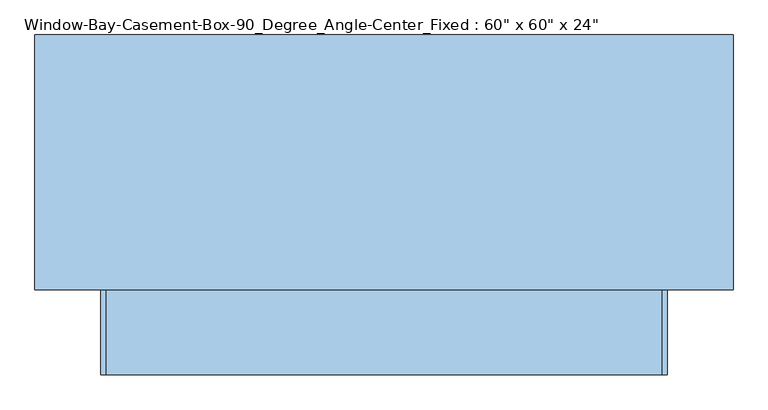
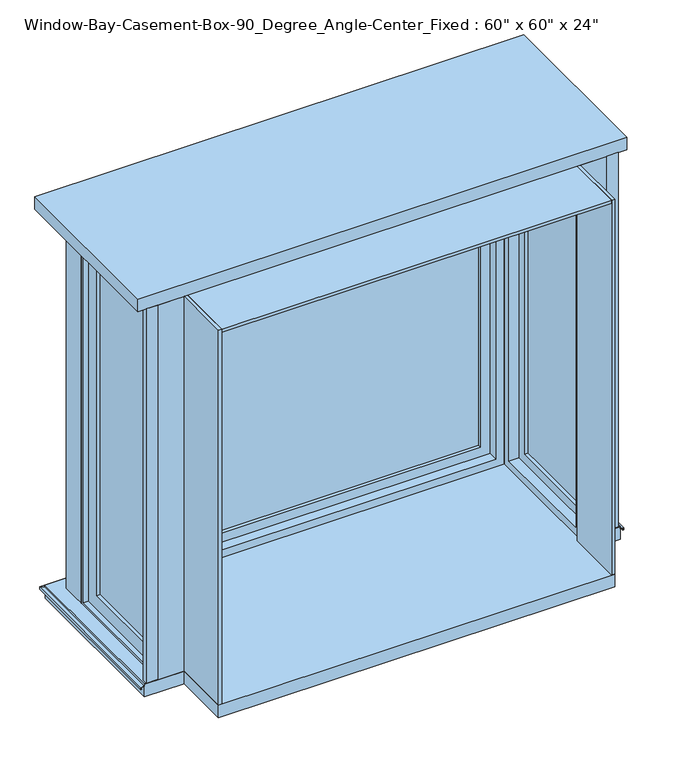
"""IFC4 building model written with IfcOpenShell, lengths in millimetres: window geometry."""

from ifc_helpers import new_model, si_unit, frame, origin, place, context, project, spatial, polyline, outline, extrude, faceted_brep, source, transform, mapped, element, save


def window_dda79932(model_context):
    return source(origin(), model_context, "Body", "SolidModel", [
        extrude(outline(polyline([(-863.6, 114.3), (-908.05, 114.3), (-908.05, 133.35), (-863.6, 133.35), (-863.6, 114.3)])), frame((0.0, 0.0, 663.1486341), z_axis=(0.0, 0.0, 1.0), x_axis=(1.0, 0.0, 0.0)), (0.0, 0.0, 1.0), 1521.2513659),
        extrude(outline(polyline([(908.05, 114.3), (863.6, 114.3), (863.6, 133.35), (908.05, 133.35), (908.05, 114.3)])), frame((0.0, 0.0, 663.1486341), z_axis=(0.0, 0.0, 1.0), x_axis=(1.0, 0.0, 0.0)), (0.0, 0.0, 1.0), 1521.2513659),
        faceted_brep([(-914.4, 114.3, 653.0697935), (-914.4, 114.3, 660.4), (-863.6, 114.3, 660.4), (-863.6, 114.3, 663.1486341), (-915.797, 114.3, 663.1486341), (-915.797, 114.3, 654.4483503), (-928.497, 114.3, 652.2089977), (-928.497, 114.3, 643.2668038), (-924.5346, 114.3, 643.2668038), (-924.5346, 114.3, 644.7270038), (-926.8968, 114.3, 644.7270038), (-926.8968, 114.3, 650.8662705), (914.4, 114.3, 653.0697935), (926.8968, 114.3, 650.8662705), (926.8968, 114.3, 644.7270038), (924.5346, 114.3, 644.7270038), (924.5346, 114.3, 643.2668038), (928.497, 114.3, 643.2668038), (928.497, 114.3, 652.2089977), (915.797, 114.3, 654.4483503), (915.797, 114.3, 663.1486341), (863.6, 114.3, 663.1486341), (863.6, 114.3, 660.4), (914.4, 114.3, 660.4), (-914.4, 774.7, 653.0697935), (-914.4, 774.7, 660.4), (914.4, 774.7, 660.4), (863.6, 723.9, 660.4), (-863.6, 723.9, 660.4), (-863.6, 723.9, 663.1486341), (863.6, 723.9, 663.1486341), (915.797, 776.097, 663.1486341), (-915.797, 776.097, 663.1486341), (-915.797, 776.097, 654.4483503), (-928.497, 788.797, 652.2089977), (-928.497, 788.797, 643.2668038), (928.497, 788.797, 643.2668038), (924.5346, 784.8346, 643.2668038), (-924.5346, 784.8346, 643.2668038), (-924.5346, 784.8346, 644.7270038), (924.5346, 784.8346, 644.7270038), (926.8968, 787.1968, 644.7270038), (-926.8968, 787.1968, 644.7270038), (-926.8968, 787.1968, 650.8662705), (914.4, 774.7, 653.0697935), (915.797, 776.097, 654.4483503), (928.497, 788.797, 652.2089977), (926.8968, 787.1968, 650.8662705)], [[[0, 1, 2, 3, 4, 5, 6, 7, 8, 9, 10, 11]], [[12, 13, 14, 15, 16, 17, 18, 19, 20, 21, 22, 23]], [[1, 0, 24, 25]], [[2, 1, 25, 26, 23, 22, 27, 28]], [[3, 2, 28, 29]], [[4, 3, 29, 30, 21, 20, 31, 32]], [[5, 4, 32, 33]], [[6, 5, 33, 34]], [[7, 6, 34, 35]], [[8, 7, 35, 36, 17, 16, 37, 38]], [[9, 8, 38, 39]], [[10, 9, 39, 40, 15, 14, 41, 42]], [[11, 10, 42, 43]], [[0, 11, 43, 24]], [[25, 24, 44, 26]], [[29, 28, 27, 30]], [[33, 32, 31, 45]], [[34, 33, 45, 46]], [[35, 34, 46, 36]], [[39, 38, 37, 40]], [[43, 42, 41, 47]], [[24, 43, 47, 44]], [[26, 44, 12, 23]], [[30, 27, 22, 21]], [[45, 31, 20, 19]], [[46, 45, 19, 18]], [[36, 46, 18, 17]], [[40, 37, 16, 15]], [[47, 41, 14, 13]], [[44, 47, 13, 12]]]),
        extrude(outline(polyline([(914.4, 774.7), (914.4, 114.3), (762.0, 114.3), (762.0, -114.3), (-762.0, -114.3), (-762.0, 114.3), (-914.4, 114.3), (-914.4, 774.7), (914.4, 774.7)])), frame((0.0, 0.0, 609.6), z_axis=(0.0, 0.0, 1.0), x_axis=(1.0, 0.0, 0.0)), (0.0, 0.0, 1.0), 50.8),
        extrude(outline(polyline([(939.8, 800.1), (939.8, 114.3), (-939.8, 114.3), (-939.8, 800.1), (939.8, 800.1)])), frame((0.0, 0.0, 2184.4), z_axis=(0.0, 0.0, 1.0), x_axis=(1.0, 0.0, 0.0)), (0.0, 0.0, 1.0), 50.8),
        extrude(outline(polyline([(-762.0, 723.9), (-762.0, 622.3), (-863.6, 622.3), (-863.6, 723.9), (-762.0, 723.9)])), frame((0.0, 0.0, 660.4), z_axis=(0.0, 0.0, 1.0), x_axis=(1.0, 0.0, 0.0)), (0.0, 0.0, 1.0), 1524.0),
        extrude(outline(polyline([(863.6, 723.9), (863.6, 622.3), (762.0, 622.3), (762.0, 723.9), (863.6, 723.9)])), frame((0.0, 0.0, 660.4), z_axis=(0.0, 0.0, 1.0), x_axis=(1.0, 0.0, 0.0)), (0.0, 0.0, 1.0), 1524.0),
        faceted_brep([(749.3, 660.4, 673.1), (749.3, 723.9, 673.1), (-749.3, 723.9, 673.1), (-749.3, 660.4, 673.1), (730.25, 622.3, 692.15), (730.25, 660.4, 692.15), (-730.25, 660.4, 692.15), (-730.25, 622.3, 692.15), (762.0, 723.9, 660.4), (762.0, 622.3, 660.4), (-762.0, 622.3, 660.4), (-762.0, 723.9, 660.4), (-749.3, 723.9, 2171.7), (-749.3, 660.4, 2171.7), (-730.25, 660.4, 2152.65), (-730.25, 622.3, 2152.65), (-762.0, 622.3, 2184.4), (-762.0, 723.9, 2184.4), (749.3, 723.9, 2171.7), (749.3, 660.4, 2171.7), (730.25, 660.4, 2152.65), (730.25, 622.3, 2152.65), (762.0, 622.3, 2184.4), (762.0, 723.9, 2184.4)], [[[0, 1, 2, 3]], [[4, 5, 6, 7]], [[8, 9, 10, 11]], [[3, 2, 12, 13]], [[7, 6, 14, 15]], [[11, 10, 16, 17]], [[13, 12, 18, 19]], [[15, 14, 20, 21]], [[17, 16, 22, 23]], [[11, 17, 23, 8], [1, 18, 12, 2]], [[19, 18, 1, 0]], [[3, 13, 19, 0], [5, 20, 14, 6]], [[21, 20, 5, 4]], [[9, 22, 16, 10], [7, 15, 21, 4]], [[23, 22, 9, 8]]]),
        extrude(outline(polyline([(2171.7, -749.3), (673.1, -749.3), (673.1, 749.3), (2171.7, 749.3), (2171.7, -749.3)]), holes=[polyline([(2114.55, 692.15), (730.25, 692.15), (730.25, -692.15), (2114.55, -692.15), (2114.55, 692.15)])]), frame((0.0, 660.4, 0.0), z_axis=(0.0, 1.0, 0.0), x_axis=(0.0, 0.0, 1.0)), (0.0, 0.0, 1.0), 44.45),
        faceted_brep([(-762.0, 146.05, 2152.65), (-800.1, 146.05, 2152.65), (-800.1, 590.55, 2152.65), (-762.0, 590.55, 2152.65), (-863.6, 114.3, 2184.4), (-762.0, 114.3, 2184.4), (-762.0, 622.3, 2184.4), (-863.6, 622.3, 2184.4), (-800.1, 127.0, 2171.7), (-863.6, 127.0, 2171.7), (-863.6, 609.6, 2171.7), (-800.1, 609.6, 2171.7), (-800.1, 590.55, 692.15), (-762.0, 590.55, 692.15), (-762.0, 622.3, 660.4), (-863.6, 622.3, 660.4), (-863.6, 609.6, 673.1), (-800.1, 609.6, 673.1), (-800.1, 146.05, 692.15), (-762.0, 146.05, 692.15), (-762.0, 114.3, 660.4), (-863.6, 114.3, 660.4), (-863.6, 127.0, 673.1), (-800.1, 127.0, 673.1)], [[[0, 1, 2, 3]], [[4, 5, 6, 7]], [[8, 9, 10, 11]], [[3, 2, 12, 13]], [[7, 6, 14, 15]], [[11, 10, 16, 17]], [[13, 12, 18, 19]], [[15, 14, 20, 21]], [[17, 16, 22, 23]], [[11, 17, 23, 8], [1, 18, 12, 2]], [[19, 18, 1, 0]], [[5, 20, 14, 6], [3, 13, 19, 0]], [[21, 20, 5, 4]], [[7, 15, 21, 4], [9, 22, 16, 10]], [[23, 22, 9, 8]]]),
        extrude(outline(polyline([(609.6, 2171.7), (609.6, 673.1), (127.0, 673.1), (127.0, 2171.7), (609.6, 2171.7)]), holes=[polyline([(184.15, 2114.55), (184.15, 730.25), (552.45, 730.25), (552.45, 2114.55), (184.15, 2114.55)])]), frame((-844.55, 0.0, 0.0), z_axis=(1.0, 0.0, 0.0), x_axis=(0.0, 1.0, 0.0)), (0.0, 0.0, 1.0), 44.45),
        faceted_brep([(800.1, 146.05, 2152.65), (762.0, 146.05, 2152.65), (762.0, 590.55, 2152.65), (800.1, 590.55, 2152.65), (863.6, 127.0, 2171.7), (800.1, 127.0, 2171.7), (800.1, 609.6, 2171.7), (863.6, 609.6, 2171.7), (762.0, 114.3, 2184.4), (863.6, 114.3, 2184.4), (863.6, 622.3, 2184.4), (762.0, 622.3, 2184.4), (762.0, 590.55, 692.15), (800.1, 590.55, 692.15), (800.1, 609.6, 673.1), (863.6, 609.6, 673.1), (863.6, 622.3, 660.4), (762.0, 622.3, 660.4), (762.0, 146.05, 692.15), (800.1, 146.05, 692.15), (800.1, 127.0, 673.1), (863.6, 127.0, 673.1), (863.6, 114.3, 660.4), (762.0, 114.3, 660.4)], [[[0, 1, 2, 3]], [[4, 5, 6, 7]], [[8, 9, 10, 11]], [[3, 2, 12, 13]], [[7, 6, 14, 15]], [[11, 10, 16, 17]], [[13, 12, 18, 19]], [[15, 14, 20, 21]], [[17, 16, 22, 23]], [[11, 17, 23, 8], [1, 18, 12, 2]], [[19, 18, 1, 0]], [[5, 20, 14, 6], [3, 13, 19, 0]], [[21, 20, 5, 4]], [[9, 22, 16, 10], [7, 15, 21, 4]], [[23, 22, 9, 8]]]),
        extrude(outline(polyline([(609.6, 2171.7), (609.6, 673.1), (127.0, 673.1), (127.0, 2171.7), (609.6, 2171.7)]), holes=[polyline([(184.15, 2114.55), (184.15, 730.25), (552.45, 730.25), (552.45, 2114.55), (184.15, 2114.55)])]), frame((800.1, 0.0, 0.0), z_axis=(1.0, 0.0, 0.0), x_axis=(0.0, 1.0, 0.0)), (0.0, 0.0, 1.0), 44.45),
        extrude(outline(polyline([(692.15, 692.15), (692.15, 685.8), (-692.15, 685.8), (-692.15, 692.15), (692.15, 692.15)])), frame((0.0, 0.0, 730.25), z_axis=(0.0, 0.0, 1.0), x_axis=(1.0, 0.0, 0.0)), (0.0, 0.0, 1.0), 1384.3),
        extrude(outline(polyline([(692.15, 679.45), (692.15, 673.1), (-692.15, 673.1), (-692.15, 679.45), (692.15, 679.45)])), frame((0.0, 0.0, 730.25), z_axis=(0.0, 0.0, 1.0), x_axis=(1.0, 0.0, 0.0)), (0.0, 0.0, 1.0), 1384.3),
        extrude(outline(polyline([(-825.5, 552.45), (-825.5, 184.15), (-831.85, 184.15), (-831.85, 552.45), (-825.5, 552.45)])), frame((0.0, 0.0, 730.25), z_axis=(0.0, 0.0, 1.0), x_axis=(1.0, 0.0, 0.0)), (0.0, 0.0, 1.0), 1384.3),
        extrude(outline(polyline([(-812.8, 552.45), (-812.8, 184.15), (-819.15, 184.15), (-819.15, 552.45), (-812.8, 552.45)])), frame((0.0, 0.0, 730.25), z_axis=(0.0, 0.0, 1.0), x_axis=(1.0, 0.0, 0.0)), (0.0, 0.0, 1.0), 1384.3),
        extrude(outline(polyline([(831.85, 552.45), (831.85, 184.15), (825.5, 184.15), (825.5, 552.45), (831.85, 552.45)])), frame((0.0, 0.0, 730.25), z_axis=(0.0, 0.0, 1.0), x_axis=(1.0, 0.0, 0.0)), (0.0, 0.0, 1.0), 1384.3),
        extrude(outline(polyline([(819.15, 552.45), (819.15, 184.15), (812.8, 184.15), (812.8, 552.45), (819.15, 552.45)])), frame((0.0, 0.0, 730.25), z_axis=(0.0, 0.0, 1.0), x_axis=(1.0, 0.0, 0.0)), (0.0, 0.0, 1.0), 1384.3),
        faceted_brep([(863.6, 127.0, 2171.7), (800.1, 127.0, 2171.7), (800.1, 609.6, 2171.7), (863.6, 609.6, 2171.7), (762.0, 114.3, 2184.4), (863.6, 114.3, 2184.4), (863.6, 622.3, 2184.4), (762.0, 622.3, 2184.4), (800.1, 146.05, 2152.65), (762.0, 146.05, 2152.65), (762.0, 590.55, 2152.65), (800.1, 590.55, 2152.65), (800.1, 609.6, 673.1), (863.6, 609.6, 673.1), (863.6, 622.3, 660.4), (762.0, 622.3, 660.4), (762.0, 590.55, 692.15), (800.1, 590.55, 692.15), (800.1, 127.0, 673.1), (863.6, 127.0, 673.1), (863.6, 114.3, 660.4), (762.0, 114.3, 660.4), (762.0, 146.05, 692.15), (800.1, 146.05, 692.15)], [[[0, 1, 2, 3]], [[4, 5, 6, 7]], [[8, 9, 10, 11]], [[3, 2, 12, 13]], [[7, 6, 14, 15]], [[11, 10, 16, 17]], [[13, 12, 18, 19]], [[15, 14, 20, 21]], [[17, 16, 22, 23]], [[1, 18, 12, 2], [11, 17, 23, 8]], [[19, 18, 1, 0]], [[5, 20, 14, 6], [3, 13, 19, 0]], [[21, 20, 5, 4]], [[7, 15, 21, 4], [9, 22, 16, 10]], [[23, 22, 9, 8]]]),
        extrude(outline(polyline([(-749.3, 114.3), (-749.3, -114.3), (-762.0, -114.3), (-762.0, 114.3), (-749.3, 114.3)])), frame((0.0, 0.0, 660.4), z_axis=(0.0, 0.0, 1.0), x_axis=(1.0, 0.0, 0.0)), (0.0, 0.0, 1.0), 1524.0),
        extrude(outline(polyline([(749.3, 114.3), (762.0, 114.3), (762.0, -114.3), (749.3, -114.3), (749.3, 114.3)])), frame((0.0, 0.0, 660.4), z_axis=(0.0, 0.0, 1.0), x_axis=(1.0, 0.0, 0.0)), (0.0, 0.0, 1.0), 1524.0),
        extrude(outline(polyline([(749.3, -114.3), (-749.3, -114.3), (-749.3, 622.3), (749.3, 622.3), (749.3, -114.3)])), frame((0.0, 0.0, 2171.7), z_axis=(0.0, 0.0, 1.0), x_axis=(1.0, 0.0, 0.0)), (0.0, 0.0, 1.0), 12.7),
    ])


if __name__ == "__main__":
    model = new_model("IFC4")
    model_context = context("Model", 3, world=origin())
    ifc_project = project(units=[si_unit("LENGTHUNIT", "METRE", prefix="MILLI")], contexts=[model_context])
    site = spatial("IfcSite", under=ifc_project)
    building = spatial("IfcBuilding", under=site)
    placement = place(None, origin())
    window_shape = window_dda79932(model_context)
    element("IfcWindow", 1, ObjectType="Window-Bay-Casement-Box-90_Degree_Angle-Center_Fixed : 60\" x 60\" x 24\"", at=placement, inside=building, context=model_context, shape_type="MappedRepresentation", body=[
        mapped(window_shape, transform((0.0, 0.0, 0.0), x_axis=(1.0, 0.0, 0.0), y_axis=(0.0, 1.0, 0.0), z_axis=(0.0, 0.0, 1.0))),
    ])
    save(model, "model.ifc")

# Revit data of these elements
# Type "Window-Bay-Casement-Box-90_Degree_Angle-Center_Fixed : 60\" x 60\" x 24\""
#   Type Mark = "29"
#   Fire Rating = "0.5h"
#   Assembly Code = "B2020100"
#   Analytic Construction = "1/8 in Pilkington single glazing"
#   Width = 5' - 0"
#   Wall Thickness [instance default] = 0' - 6"
#   Visual Light Transmittance = 0.9
#   Trim Width = 5' - 8"
#   Trim Height = 5' - 0"
#   Thermal Resistance (R) = 1.5394 (h·ft²·°F)/BTU
#   Solar Heat Gain Coefficient = 0.86
#   Rough Width = 5' - 0 1/2"
#   Rough Height = 5' - 0 1/2"
#   Height 1 = 5' - 2"
#   Height = 5' - 0"
#   Heat Transfer Coefficient (U) = 0.6496 BTU/(h·ft²·°F)
#   Depth = 2' - 0"
#   Default Sill Height = 2' - 0"
#   Side Muntin Visibility = yes
#   Center Muntin Visibility = yes
#   Interior Trim Visibility [instance default] = yes
#   Exterior Trim Visibility [instance default] = yes
#   Side Muntin Pattern = Muntin Pattern_2x2 : Muntin Pattern_2x2
#   Center Muntin Pattern = Muntin Pattern_2x2 : Muntin Pattern_2x2
#   Interior Trim Material = Wood - Stained
#   Exterior Trim Material = Clad - White
#   Exterior Trim = element 424880
#   Interior Trim = Trim-Window-Interior-Flat : Picture Frame
#   Interior Frame Material = Wood - Stained
#   Glass Panel Material = Glass
#   Exterior Frame Material = Clad - White
#   Wall Closure = (empty or 0)
# Element 1 (IfcWindow, "Window-Bay-Casement-Box-90_Degree_Angle-Center_Fixed : 60\" x 60\" x 24\"")
#   Wall Thickness = 0' - 9"
#   Materials on its faces: "Clad - White", "Wood - Stained", "Glass"
# Materials
#   "Wood - Stained": class "Wood", colour RGB 224 178 126, transparency 0, Cost = 0
#   "Clad - White": class "Wood", colour RGB 242 242 238, transparency 0, Cost = 0
#   "Glass": class "Glass", colour RGB 0 128 192, transparency 0.75, Description = "Soda Lime Glass", Cost = 0
